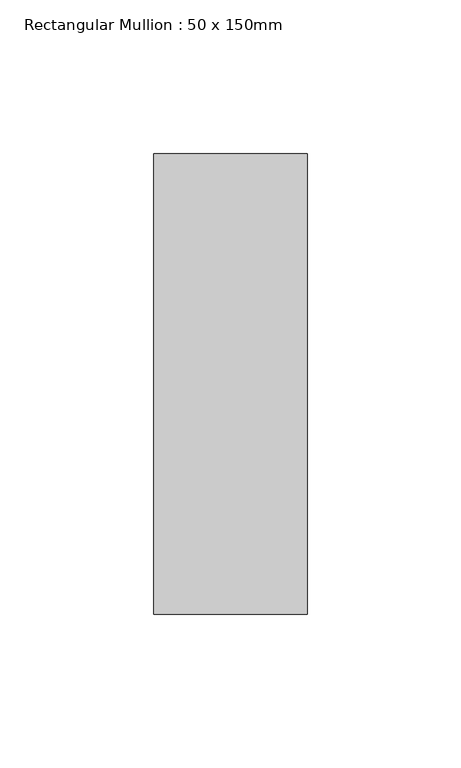
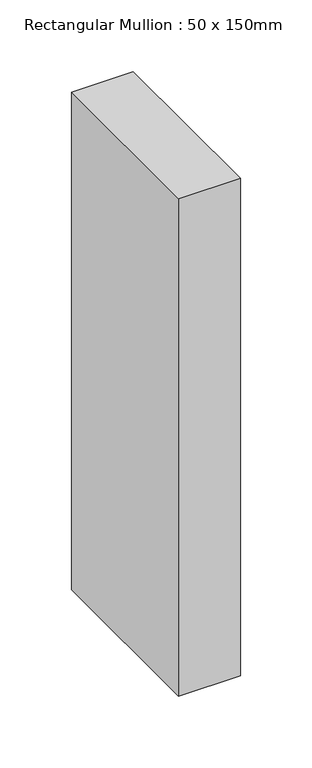
"""IFC4 building model written with IfcOpenShell, lengths in millimetres: member geometry, Rectangular Mullion : 50 x 150mm."""

from ifc_helpers import new_model, si_unit, frame, origin, place, context, project, spatial, polyline, outline, extrude, source, transform, mapped, element, save


def rectangular_mullion_50_x_150mm_129a33a7(model_context):
    return source(origin(), model_context, "Body", "SweptSolid", [
        extrude(outline(polyline([(25.0, 75.0), (25.0, -75.0), (-25.0, -75.0), (-25.0, 75.0), (25.0, 75.0)])), frame((0.0, 0.0, -425.0), z_axis=(0.0, 0.0, 1.0), x_axis=(1.0, 0.0, 0.0)), (0.0, 0.0, 1.0), 425.0),
    ])


if __name__ == "__main__":
    model = new_model("IFC4")
    model_context = context("Model", 3, world=origin())
    ifc_project = project(units=[si_unit("LENGTHUNIT", "METRE", prefix="MILLI")], contexts=[model_context])
    site = spatial("IfcSite", under=ifc_project)
    building = spatial("IfcBuilding", under=site)
    placement = place(None, origin())
    rectangular_mullion_50_x_150mm_shape = rectangular_mullion_50_x_150mm_129a33a7(model_context)
    element("IfcMember", 1, ObjectType="Rectangular Mullion : 50 x 150mm", at=placement, inside=building, context=model_context, shape_type="MappedRepresentation", body=[
        mapped(rectangular_mullion_50_x_150mm_shape, transform((0.0, 0.0, 0.0), x_axis=(1.0, 0.0, 0.0), y_axis=(0.0, 1.0, 0.0), z_axis=(0.0, 0.0, 1.0))),
    ])
    save(model, "model.ifc")

# Revit data of these elements
# Type "Rectangular Mullion : 50 x 150mm"
#   built-in parameter 1007304 = 0.492126 (stored number, unit not read)
#   built-in parameter 1007301 = 0.082021 (stored number, unit not read)
#   built-in parameter 1007300 = 0.082021 (stored number, unit not read)
# Element 1 (IfcMember, "Rectangular Mullion : 50 x 150mm")
#   Materials on its faces: "Aluminium"
# Materials
#   "Aluminium": class "Metal", colour RGB 247 247 247, transparency 0, Description = "Aluminium 6061", Cost = 0
